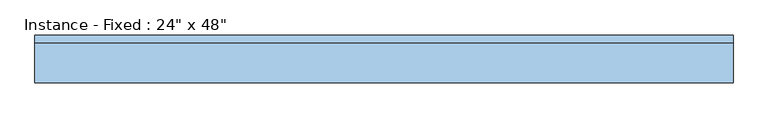
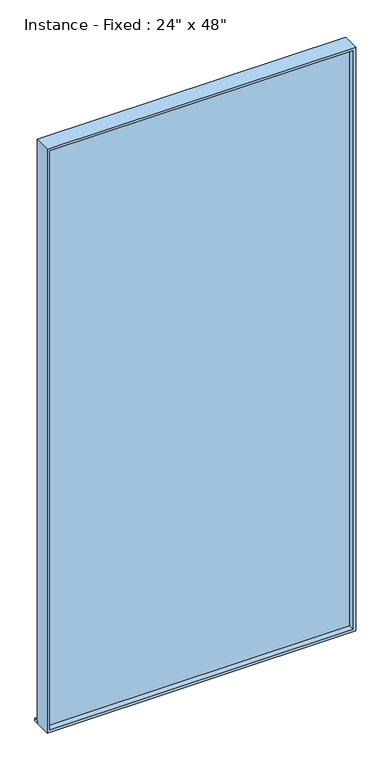
"""IFC4 building model written with IfcOpenShell, lengths in millimetres: window geometry."""

from ifc_helpers import new_model, si_unit, frame, origin, place, context, project, spatial, polyline, outline, extrude, source, transform, mapped, element, save


def window_2382273a(model_context):
    return source(origin(), model_context, "Body", "SweptSolid", [
        extrude(outline(polyline([(-1104.9, 127.0), (1028.7, 127.0), (1028.7, 101.6), (-1104.9, 101.6), (-1104.9, 127.0)])), frame((0.0, 0.0, 914.4), z_axis=(0.0, 0.0, 1.0), x_axis=(1.0, 0.0, 0.0)), (0.0, 0.0, 1.0), 19.05),
        extrude(outline(polyline([(1009.65, 22.225), (-1085.85, 22.225), (-1085.85, 34.925), (1009.65, 34.925), (1009.65, 22.225)])), frame((0.0, 0.0, 933.45), z_axis=(0.0, 0.0, 1.0), x_axis=(1.0, 0.0, 0.0)), (0.0, 0.0, 1.0), 4229.1),
        extrude(outline(polyline([(5181.6, 1028.7), (5181.6, -1104.9), (914.4, -1104.9), (914.4, 1028.7), (5181.6, 1028.7)]), holes=[polyline([(5162.55, 1009.65), (933.45, 1009.65), (933.45, -1085.85), (5162.55, -1085.85), (5162.55, 1009.65)])]), frame((0.0, -19.05, 0.0), z_axis=(0.0, 1.0, 0.0), x_axis=(0.0, 0.0, 1.0)), (0.0, 0.0, 1.0), 120.65),
    ])


if __name__ == "__main__":
    model = new_model("IFC4")
    model_context = context("Model", 3, world=origin())
    ifc_project = project(units=[si_unit("LENGTHUNIT", "METRE", prefix="MILLI")], contexts=[model_context])
    site = spatial("IfcSite", under=ifc_project)
    building = spatial("IfcBuilding", under=site)
    placement = place(None, origin())
    window_shape = window_2382273a(model_context)
    element("IfcWindow", 1, ObjectType="Instance - Fixed : 24\" x 48\"", at=placement, inside=building, context=model_context, shape_type="MappedRepresentation", body=[
        mapped(window_shape, transform((0.0, 0.0, 0.0), x_axis=(1.0, 0.0, 0.0), y_axis=(0.0, 1.0, 0.0), z_axis=(0.0, 0.0, 1.0))),
    ])
    save(model, "model.ifc")

# Revit data of these elements
# Type "Instance - Fixed : 24\" x 48\""
#   Type Mark = "10"
#   Construction Type Id = "GSP4R"
#   Assembly Code = "B2020100"
#   Analytic Construction = "1/8 in Pilkington single glazing"
#   Visual Light Transmittance = 0.9
#   Thermal Resistance (R) = 0.8466 (h·ft²·°F)/BTU
#   Solar Heat Gain Coefficient = 0.86
#   Heat Transfer Coefficient (U) = 1.1812 BTU/(h·ft²·°F)
#   Height [instance default] = 4' - 0"
#   Default Sill Height = 3' - 0"
#   Width [instance default] = 2' - 0"
#   Window Inset = 0' - 2"
#   Define Thermal Properties by = 1
#   Glass Pane Material = Glass
#   Sash Material = Iron, Ductile
#   Wall Closure = (empty or 0)
# Element 1 (IfcWindow, "Instance - Fixed : 24\" x 48\"")
#   Height = 14' - 0"
#   Width = 7' - 0"
#   Materials on its faces: "Iron, Ductile", "Glass"
# Materials
#   "Glass": class "Glass", colour RGB 0 128 192, transparency 0.75, Description = "Soda Lime Glass", Cost = 0
#   "Iron, Ductile": class "Metal", colour RGB 0 0 0, transparency 0, Description = "Ductile cast iron", Cost = 0
